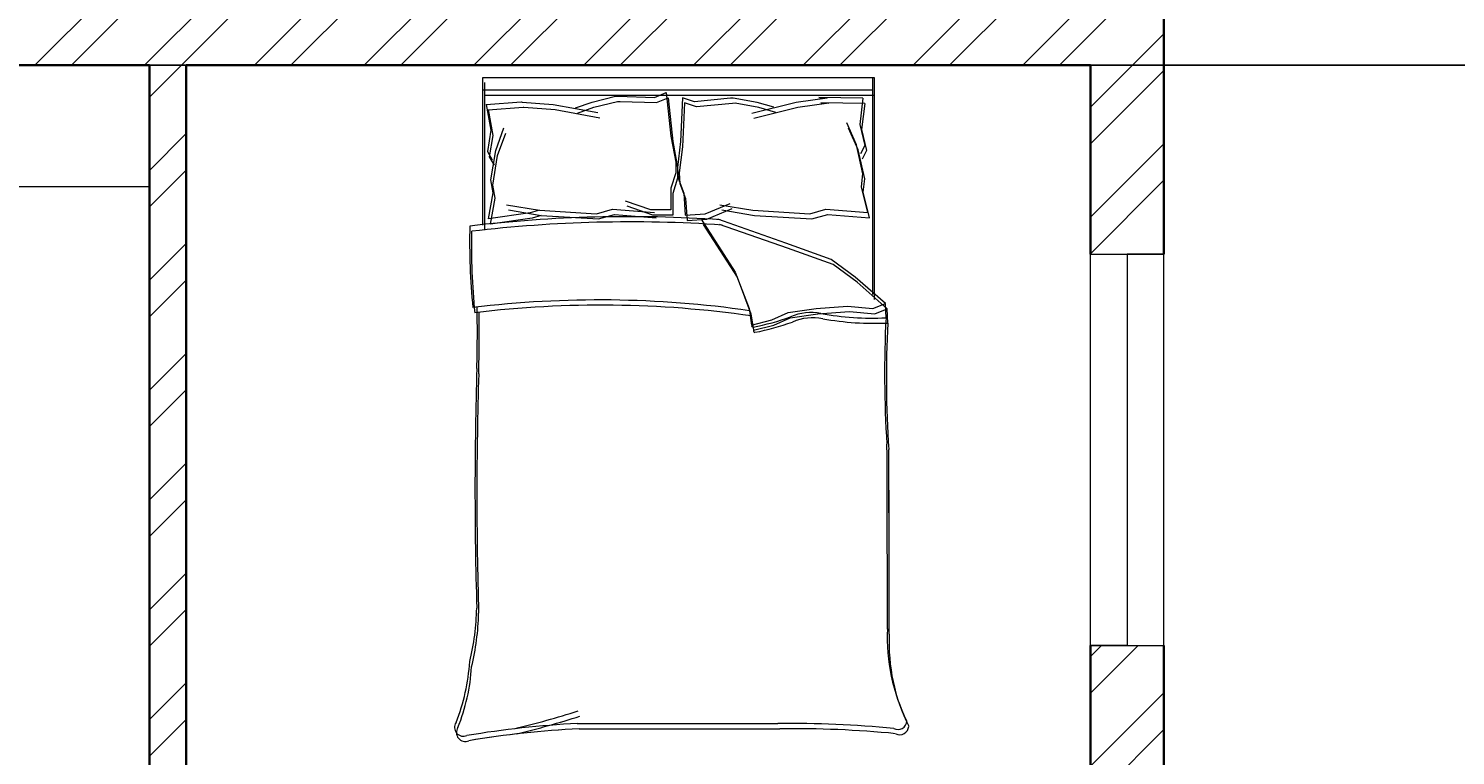
# Model space of a CAD drawing. Units: inches. Extents: x 2552 to 3217, y 1417 to 2737.
# Tile 11 of 25: x 2710 to 2885, y 2302 to 2392. Entities that reach past the tile are written whole.
import ezdxf

# ---------------------------------------------------------------- set-up
doc = ezdxf.new("R2010")
doc.units = ezdxf.units.IN
for name, color, linetype, lineweight in [('A-ANNO-DIMS', 2, 'Continuous', 18), ('A-FLOR-CASE', 9, 'Continuous', 18), ('A-FURN', 8, 'Continuous', 13), ('A-GLAZ', 161, 'Continuous', 18), ('A-WALL', 7, 'Continuous', 35), ('A-WALL-PATT', 217, 'Continuous', 13)]:
    doc.layers.add(name, color=color, linetype=linetype, lineweight=lineweight)
doc.styles.get("Standard").update_dxf_attribs({"font": 'arial.ttf'})
doc.dimstyles.get("Standard").update_dxf_attribs({"dimtxt": 0.18, "dimasz": 0.18, "dimexe": 0.18, "dimexo": 0.0625, "dimgap": 0.09, "dimtad": 0, "dimtih": 1, "dimtoh": 1, "dimdec": 4, "dimzin": 0, "dimdsep": 46, "dimtxsty": 'Standard', "dimcen": 0.09, "dimadec": 0, "dimazin": 0, "dimtfac": 1, "dimtdec": 4, "dimtofl": 0, "dimtmove": 0, "dimatfit": 3, "dimfxl": 1, "dimtolj": 1, "dimtzin": 0, "dimarcsym": 0})

# ---------------------------------------------------------------- blocks, each defined once
blk = doc.blocks.new('BED-DOUBLE')
for p, q in [((3.47, 63.33), (3.47, 81.44)), ((3.47, 81.44), (51.49, 81.44)), ((3.48, 63.33), (3.48, 81.44)), ((3.7, 62.69), (3.7, 80.8)), ((3.7, 62.69), (3.7, 80.8)), ((51.27, 81.44), (51.27, 54.83)), ((51.27, 81.44), (51.27, 54.83)), ((51.49, 81.44), (51.49, 80.8)), ((51.49, 80.8), (51.49, 54.19)), ((51.49, 80.8), (51.49, 54.19)), ((3.47, 79.91), (51.27, 79.91)), ((3.48, 79.91), (51.27, 79.91)), ((3.7, 79.27), (51.49, 79.27)), ((3.7, 79.27), (51.49, 79.27)), ((16.88, 78.42), (19.77, 79.14)), ((16.88, 78.42), (19.77, 79.14)), ((19.77, 79.14), (20.09, 79.14)), ((19.77, 79.14), (20.09, 79.14)), ((20.09, 79.14), (24.54, 78.99)), ((20.09, 79.14), (24.54, 78.99)), ((24.54, 78.99), (25.98, 79.57)), ((24.54, 78.99), (25.98, 79.57)), ((24.77, 78.36), (26.21, 78.93)), ((24.77, 78.36), (26.21, 78.93)), ((25.98, 79.57), (26.56, 74.22)), ((25.98, 79.57), (26.56, 74.22)), ((26.21, 78.93), (26.79, 73.58)), ((26.21, 78.93), (26.79, 73.58)), ((27.98, 78.95), (27.73, 73.58)), ((27.98, 78.95), (27.73, 73.58)), ((29.46, 78.46), (27.98, 78.95)), ((29.46, 78.46), (27.98, 78.95)), ((33.88, 78.89), (29.46, 78.46)), ((33.88, 78.89), (29.46, 78.46)), ((34.2, 78.91), (33.88, 78.89)), ((34.2, 78.91), (33.88, 78.89)), ((37.14, 78.36), (34.2, 78.91)), ((37.14, 78.36), (34.2, 78.91)), ((45.71, 78.9), (41.91, 78.37)), ((45.71, 78.9), (41.91, 78.37)), ((50.11, 78.89), (44.71, 78.98)), ((44.71, 78.98), (45.71, 78.9)), ((50.11, 78.89), (44.71, 78.98)), ((44.71, 78.98), (45.71, 78.9)), ((50.11, 78.89), (49.73, 75.68)), ((50.11, 78.89), (49.73, 75.68)), ((3.89, 78.13), (4.47, 74.95)), ((3.89, 78.13), (4.47, 74.95)), ((3.9, 78.11), (8.18, 78.43)), ((3.9, 78.11), (8.18, 78.43)), ((4.12, 77.49), (4.7, 74.31)), ((4.12, 77.49), (4.7, 74.31)), ((4.13, 77.47), (8.41, 77.8)), ((4.13, 77.47), (8.41, 77.8)), ((8.18, 78.43), (8.28, 78.42)), ((8.18, 78.43), (8.28, 78.42)), ((8.28, 78.42), (12.11, 78.13)), ((8.28, 78.42), (12.11, 78.13)), ((8.41, 77.8), (8.51, 77.78)), ((8.41, 77.8), (8.51, 77.78)), ((8.51, 77.78), (12.34, 77.49)), ((8.51, 77.78), (12.34, 77.49)), ((12.11, 78.13), (17.6, 77.12)), ((12.11, 78.13), (17.6, 77.12)), ((12.34, 77.49), (17.83, 76.48)), ((12.34, 77.49), (17.83, 76.48)), ((14.85, 77.69), (16.88, 78.42)), ((14.85, 77.69), (16.88, 78.42)), ((15.08, 77.05), (17.11, 77.78)), ((15.08, 77.05), (17.11, 77.78)), ((17.11, 77.78), (20, 78.5)), ((17.11, 77.78), (20, 78.5)), ((20, 78.5), (20.32, 78.5)), ((20, 78.5), (20.32, 78.5)), ((20.32, 78.5), (24.77, 78.36)), ((20.32, 78.5), (24.77, 78.36)), ((28.21, 78.31), (27.96, 72.94)), ((28.21, 78.31), (27.96, 72.94)), ((29.68, 77.83), (28.21, 78.31)), ((29.68, 77.83), (28.21, 78.31)), ((34.11, 78.25), (29.68, 77.83)), ((34.11, 78.25), (29.68, 77.83)), ((34.43, 78.27), (34.11, 78.25)), ((34.43, 78.27), (34.11, 78.25)), ((37.36, 77.73), (34.43, 78.27)), ((37.36, 77.73), (34.43, 78.27)), ((41.91, 78.37), (36.49, 77.02)), ((41.91, 78.37), (36.5, 77.02)), ((42.14, 77.73), (36.72, 76.38)), ((42.14, 77.73), (36.72, 76.38)), ((39.2, 77.77), (37.14, 78.36)), ((39.2, 77.77), (37.14, 78.36)), ((39.43, 77.13), (37.36, 77.73)), ((39.43, 77.13), (37.36, 77.73)), ((45.94, 78.26), (42.14, 77.73)), ((45.94, 78.26), (42.14, 77.73)), ((50.34, 78.25), (44.94, 78.34)), ((44.94, 78.34), (45.94, 78.26)), ((50.34, 78.25), (44.94, 78.34)), ((44.94, 78.34), (45.94, 78.26)), ((50.34, 78.25), (49.96, 75.04)), ((50.34, 78.25), (49.96, 75.04)), ((49.31, 73.19), (48.13, 75.86)), ((49.31, 73.19), (48.13, 75.86)), ((49.73, 75.68), (50.33, 73.1)), ((49.73, 75.68), (50.33, 73.1)), ((4.47, 74.95), (4.04, 72.34)), ((4.47, 74.95), (4.04, 72.34)), ((4.7, 74.31), (4.27, 71.7)), ((4.7, 74.31), (4.27, 71.7)), ((5.05, 72.49), (6.06, 75.24)), ((5.05, 72.49), (6.06, 75.24)), ((5.28, 71.85), (6.29, 74.6)), ((5.28, 71.85), (6.29, 74.6)), ((26.56, 74.22), (27.14, 71.04)), ((26.56, 74.22), (27.14, 71.04)), ((26.79, 73.58), (27.37, 70.4)), ((26.79, 73.58), (27.37, 70.4)), ((27.73, 73.58), (27.35, 70.37)), ((27.73, 73.58), (27.35, 70.37)), ((49.54, 72.55), (48.36, 75.23)), ((49.54, 72.55), (48.36, 75.23)), ((49.96, 75.04), (50.56, 72.47)), ((49.96, 75.04), (50.56, 72.47)), ((4.04, 72.34), (4.62, 71.33)), ((4.04, 72.34), (4.62, 71.33)), ((4.47, 68.87), (5.05, 72.49)), ((4.47, 68.87), (5.05, 72.49)), ((4.7, 68.23), (5.28, 71.85)), ((4.7, 68.23), (5.28, 71.85)), ((27.96, 72.94), (27.58, 69.73)), ((27.96, 72.94), (27.58, 69.73)), ((50.11, 69.61), (49.31, 73.19)), ((50.11, 69.61), (49.31, 73.19)), ((50.34, 68.98), (49.54, 72.55)), ((50.34, 68.98), (49.54, 72.55)), ((50.33, 73.1), (49.81, 72.06)), ((50.33, 73.1), (49.81, 72.06)), ((50.56, 72.47), (50.04, 71.42)), ((50.56, 72.47), (50.04, 71.42)), ((4.27, 71.7), (4.85, 70.69)), ((4.27, 71.7), (4.85, 70.69)), ((27.14, 71.04), (27.14, 69.74)), ((27.14, 71.04), (27.14, 69.74)), ((27.35, 70.37), (27.44, 69.07)), ((27.35, 70.37), (27.44, 69.07)), ((27.37, 70.4), (27.37, 69.1)), ((27.37, 70.4), (27.37, 69.1)), ((4.76, 67.28), (4.47, 68.87)), ((4.76, 67.28), (4.47, 68.87)), ((27.14, 69.74), (26.56, 67.86)), ((27.14, 69.74), (26.56, 67.86)), ((27.37, 69.1), (26.79, 67.22)), ((27.37, 69.1), (26.79, 67.22)), ((27.44, 69.07), (28.13, 67.23)), ((27.44, 69.07), (28.13, 67.23)), ((27.58, 69.73), (27.66, 68.43)), ((27.58, 69.73), (27.66, 68.43)), ((27.66, 68.43), (28.36, 66.59)), ((27.66, 68.43), (28.36, 66.59)), ((49.92, 68.01), (50.11, 69.61)), ((49.92, 68.01), (50.11, 69.61)), ((50.15, 67.37), (50.34, 68.98)), ((50.15, 67.37), (50.34, 68.98)), ((4.18, 64.1), (4.76, 67.28)), ((4.18, 64.1), (4.76, 67.28)), ((4.41, 63.46), (4.99, 66.64)), ((4.41, 63.46), (4.99, 66.64)), ((4.99, 66.64), (4.7, 68.23)), ((4.99, 66.64), (4.7, 68.23)), ((26.56, 67.86), (26.56, 65.18)), ((26.56, 67.86), (26.56, 65.18)), ((26.79, 67.22), (26.79, 64.54)), ((26.79, 67.22), (26.79, 64.54)), ((28.13, 67.23), (28.3, 64.55)), ((28.13, 67.23), (28.3, 64.55)), ((28.36, 66.59), (28.53, 63.91)), ((28.36, 66.59), (28.53, 63.91)), ((50.7, 64.87), (49.92, 68.01)), ((50.7, 64.87), (49.92, 68.01)), ((50.93, 64.23), (50.15, 67.37)), ((50.93, 64.23), (50.15, 67.37)), ((9.28, 64.83), (4.18, 64.1)), ((9.28, 64.83), (4.18, 64.1)), ((6.38, 65.81), (10.41, 65.15)), ((6.38, 65.81), (10.41, 65.15)), ((6.61, 65.18), (10.64, 64.51)), ((6.61, 65.18), (10.64, 64.51)), ((10.41, 65.15), (9.28, 64.83)), ((10.41, 65.15), (9.28, 64.83)), ((10.41, 65.15), (17.42, 64.72)), ((10.41, 65.15), (17.42, 64.72)), ((17.42, 64.72), (19.38, 65.27)), ((17.42, 64.72), (19.38, 65.27)), ((19.38, 65.27), (24.52, 64.87)), ((19.38, 65.27), (24.52, 64.87)), ((24.1, 65.18), (20.96, 66.27)), ((24.1, 65.18), (20.96, 66.27)), ((24.33, 64.54), (21.19, 65.63)), ((24.33, 64.54), (21.19, 65.63)), ((26.56, 65.18), (24.1, 65.18)), ((26.56, 65.18), (24.1, 65.18)), ((30.75, 64.7), (33.82, 65.99)), ((30.75, 64.7), (33.82, 65.99)), ((30.98, 64.06), (34.05, 65.35)), ((30.98, 64.06), (34.05, 65.35)), ((32.56, 65.81), (36.6, 65.15)), ((32.56, 65.81), (36.6, 65.15)), ((32.79, 65.18), (36.82, 64.51)), ((32.79, 65.18), (36.82, 64.51)), ((36.6, 65.15), (43.61, 64.72)), ((36.6, 65.15), (43.61, 64.72)), ((43.61, 64.72), (45.57, 65.27)), ((43.61, 64.72), (45.57, 65.27)), ((45.57, 65.27), (50.7, 64.87)), ((45.57, 65.27), (50.7, 64.87)), ((9.51, 64.19), (4.41, 63.46)), ((9.51, 64.19), (4.41, 63.46)), ((10.64, 64.51), (9.51, 64.19)), ((10.64, 64.51), (9.51, 64.19)), ((10.64, 64.51), (17.65, 64.08)), ((10.64, 64.51), (17.65, 64.08)), ((17.65, 64.08), (19.61, 64.63)), ((17.65, 64.08), (19.61, 64.63)), ((19.61, 64.63), (24.74, 64.23)), ((19.61, 64.63), (24.74, 64.23)), ((26.79, 64.54), (24.33, 64.54)), ((26.79, 64.54), (24.33, 64.54)), ((28.3, 64.55), (30.75, 64.7)), ((28.3, 64.55), (30.75, 64.7)), ((28.53, 63.91), (30.98, 64.06)), ((28.53, 63.91), (30.98, 64.06)), ((30.26, 64.06), (34.45, 57.57)), ((30.26, 64.06), (34.45, 57.57)), ((30.49, 63.42), (34.68, 56.93)), ((30.49, 63.42), (34.68, 56.93)), ((40.64, 61.13), (32.31, 64.06)), ((40.64, 61.13), (32.31, 64.06)), ((40.87, 60.49), (32.53, 63.42)), ((40.87, 60.49), (32.53, 63.42)), ((36.82, 64.51), (43.83, 64.08)), ((36.82, 64.51), (43.83, 64.08)), ((43.83, 64.08), (45.79, 64.63)), ((43.83, 64.08), (45.79, 64.63)), ((45.79, 64.63), (50.93, 64.23)), ((45.79, 64.63), (50.93, 64.23)), ((46.22, 59.11), (40.64, 61.13)), ((46.22, 59.11), (40.64, 61.13)), ((46.45, 58.48), (40.87, 60.49)), ((46.45, 58.48), (40.87, 60.49)), ((49.16, 56.95), (46.22, 59.11)), ((49.16, 56.95), (46.22, 59.11)), ((49.39, 56.31), (46.45, 58.48)), ((49.39, 56.31), (46.45, 58.48)), ((34.45, 57.57), (36.15, 53.08)), ((34.45, 57.57), (36.15, 53.08)), ((34.68, 56.93), (36.38, 52.44)), ((34.68, 56.93), (36.38, 52.44)), ((52.87, 53.7), (49.16, 56.95)), ((52.87, 53.7), (49.16, 56.95)), ((53.1, 53.06), (49.39, 56.31)), ((53.1, 53.06), (49.39, 56.31)), ((36.15, 53.08), (36.46, 51.07)), ((36.15, 53.08), (36.46, 51.07)), ((38.94, 51.69), (40.95, 52.61)), ((38.94, 51.69), (40.95, 52.61)), ((40.95, 52.61), (44.36, 53.08)), ((40.95, 52.61), (44.36, 53.08)), ((44.36, 53.08), (48.23, 53.39)), ((44.36, 53.08), (48.23, 53.39)), ((44.59, 52.44), (48.46, 52.75)), ((44.59, 52.44), (48.46, 52.75)), ((48.23, 53.39), (51.33, 53.08)), ((48.23, 53.39), (51.33, 53.08)), ((48.46, 52.75), (51.56, 52.44)), ((48.46, 52.75), (51.56, 52.44)), ((51.33, 53.08), (52.87, 53.7)), ((51.33, 53.08), (52.87, 53.7)), ((51.56, 52.44), (53.1, 53.06)), ((51.56, 52.44), (53.1, 53.06)), ((52.95, 51.95), (52.87, 53.7, 3.87)), ((52.95, 51.95), (52.87, 53.7, 3.87)), ((53.18, 51.31), (53.1, 53.06, 3.87)), ((53.18, 51.31), (53.1, 53.06, 3.87)), ((36.38, 52.44), (36.69, 50.43)), ((36.38, 52.44), (36.69, 50.43)), ((36.46, 51.07), (38.94, 51.69)), ((36.46, 51.07), (38.94, 51.69)), ((36.69, 50.43), (39.17, 51.05)), ((36.69, 50.43), (39.17, 51.05)), ((39.17, 51.05), (41.18, 51.97)), ((39.17, 51.05), (41.18, 51.97)), ((41.18, 51.97), (44.59, 52.44)), ((41.18, 51.97), (44.59, 52.44)), ((15.06, 2.2), (39.68, 2.2)), ((15.06, 2.2), (39.68, 2.2)), ((15.29, 1.56), (39.91, 1.56)), ((15.29, 1.56), (39.91, 1.56))]:
    blk.add_line(p, q)
for centre, radius, start, end in [((85.16, 61.35), 83.31, 178.7218, 185.604), ((85.16, 61.35), 83.31, 178.7218, 185.604), ((21.36, -100.61), 164.97, 86.0865, 96.7821), ((21.36, -100.61), 164.97, 86.0865, 96.7821), ((21.59, -101.25), 164.97, 86.0865, 96.7821), ((21.59, -101.25), 164.97, 86.0865, 96.7821), ((85.39, 60.71), 83.31, 178.7218, 185.604), ((85.39, 60.71), 83.31, 178.7218, 185.604), ((17.76, -74.87), 129.02, 81.7845, 96.9006), ((17.76, -74.87), 129.02, 81.7845, 96.9006), ((17.98, -75.51), 129.02, 81.7845, 96.9006), ((17.98, -75.51), 129.02, 81.7845, 96.9006), ((-167.31, 50.27), 170.11, 358.4762, 1.0082), ((-167.31, 50.27), 170.11, 358.4762, 1.0082), ((-167.08, 49.63), 170.11, 358.4762, 1.0082), ((-167.08, 49.63), 170.11, 358.4762, 1.0082), ((43.74, 46.38), 6.22, 78.6608, 113.7384), ((43.74, 46.38), 6.22, 78.6608, 113.7384), ((36.64, 51), 0.185, 160.2464, 271.1377), ((36.64, 51), 0.185, 160.2464, 271.1377), ((31.15, 79.96), 29.65, 280.6617, 289.8806), ((31.15, 79.96), 29.65, 280.6617, 289.8806), ((31.38, 79.32), 29.65, 280.6617, 289.8806), ((31.38, 79.32), 29.65, 280.6617, 289.8806), ((43.97, 45.74), 6.22, 78.6608, 113.7384), ((43.97, 45.74), 6.22, 78.6608, 113.7384), ((51.33, 88.1), 36.18, 259.8763, 272.5657), ((51.33, 88.1), 36.18, 259.8763, 272.5657), ((51.56, 87.46), 36.18, 259.8763, 272.5657), ((51.56, 87.46), 36.18, 259.8763, 272.5657), ((182.27, 45.13), 129.5, 176.9791, 183.8365), ((182.27, 45.13), 129.5, 176.9791, 183.8365), ((182.49, 44.49), 129.5, 176.9791, 183.8365), ((182.49, 44.49), 129.5, 176.9791, 183.8365), ((36.86, 50.36), 0.185, 160.2464, 271.1377), ((36.86, 50.36), 0.185, 160.2464, 271.1377), ((484.82, 30.83), 482.31, 178.2277, 181.7185), ((484.82, 30.83), 482.31, 178.2277, 181.7185), ((485.05, 30.19), 482.31, 178.2277, 181.7185), ((485.05, 30.19), 482.31, 178.2277, 181.7185), ((-4508.74, 13.62), 4561.86, 0.00217, 0.28689), ((-4508.74, 13.62), 4561.86, 0.00217, 0.28689), ((-4508.51, 12.98), 4561.86, 0.00217, 0.28689), ((-4508.52, 12.98), 4561.86, 0.00217, 0.28689), ((-26.9, 16.93), 29.63, 346.0648, 358.9113), ((-26.9, 16.93), 29.63, 346.0648, 358.9113), ((-26.67, 16.29), 29.63, 346.0648, 358.9113), ((-26.67, 16.29), 29.63, 346.0648, 358.9113), ((76.16, 12.78), 23.07, 177.4714, 206.4681), ((76.16, 12.78), 23.07, 177.4714, 206.4681), ((76.39, 12.14), 23.07, 177.4714, 206.4681), ((76.39, 12.14), 23.07, 177.4714, 206.4681), ((-21.66, 11.17), 23.56, 337.9751, 356.652), ((-21.66, 11.17), 23.56, 337.9751, 356.652), ((-21.43, 10.53), 23.56, 337.9751, 356.652), ((-21.43, 10.53), 23.56, 337.9751, 356.652), ((-17.22, 105.16), 106.46, 283.3832, 287.7053), ((-17.22, 105.16), 106.46, 283.3832, 287.7053), ((1.09, 1.73), 1.09, 146.1736, 293.4781), ((1.09, 1.73), 1.09, 146.1736, 293.4781), ((21.43, -119.39), 121.76, 92.9958, 99.4091), ((21.43, -119.39), 121.76, 92.9958, 99.4091), ((-16.99, 104.52), 106.46, 283.3832, 287.7053), ((-16.99, 104.52), 106.46, 283.3832, 287.7053), ((41.15, -130.83), 133.04, 84.4998, 90.6351), ((41.15, -130.83), 133.04, 84.4998, 90.6351), ((54.41, 2.57), 1.1, 242.6588, 356.02), ((54.41, 2.57), 1.1, 242.6588, 356.02), ((54.64, 1.93), 1.1, 242.6588, 356.02), ((54.64, 1.93), 1.1, 242.6588, 356.02), ((1.32, 1.09), 1.09, 146.1736, 293.4781), ((1.32, 1.09), 1.09, 146.1736, 293.4781), ((21.66, -120.03), 121.76, 92.9958, 99.4091), ((21.65, -120.03), 121.76, 92.9958, 99.4091), ((41.38, -131.47), 133.04, 84.4998, 90.6351), ((41.38, -131.47), 133.04, 84.4998, 90.6351)]:
    blk.add_arc(centre, radius, start, end)
blk = doc.blocks.new('WIN-48')
for p, q in [((4.5, 48), (0, 48)), ((0, 48), (9, 48)), ((0, 48), (0, 0)), ((4.5, 0), (4.5, 48)), ((9, 48), (9, 0)), ((0, 0), (9, 0)), ((9, 0), (4.5, 0))]:
    blk.add_line(p, q)
blk = doc.blocks.new('*D64')
at = {"layer": 'A-ANNO-DIMS', "color": 0, "lineweight": -2, "transparency": 16777216}
for p, q in [((2646.35, 1551.58), (2646.35, 2709.49)), ((2646.53, 2709.31), (2802.77, 2709.31)), ((2959.93, 2709.31), (2803.69, 2709.31)), ((2960.11, 1551.58), (2960.11, 2709.49))]:
    blk.add_line(p, q, dxfattribs=at)
at = {"layer": 'A-ANNO-DIMS', "color": 0, "transparency": 16777216}
for points in [[(2646.53, 2709.34), (2646.53, 2709.28), (2646.35, 2709.31)], [(2959.93, 2709.34), (2959.93, 2709.28), (2960.11, 2709.31)]]:
    blk.add_solid(points, dxfattribs=at)
at = {"layer": 'Defpoints', "color": 0, "transparency": 16777216}
for p in [(2960.11, 2709.31), (2646.35, 1551.51), (2960.11, 1551.51)]:
    blk.add_point(p, dxfattribs=at)
at = {"layer": 'A-ANNO-DIMS', "color": 0, "transparency": 16777216, "insert": (2803.23, 2709.31), "char_height": 0.18, "attachment_point": 5}
blk.add_mtext('\\A1;313.76', dxfattribs=at)
blk = doc.blocks.new('*D69')
at = {"layer": 'A-ANNO-DIMS', "color": 0, "lineweight": -2, "transparency": 16777216}
for p, q in [((2908.79, 2403.41), (2577.37, 2403.41)), ((2577.55, 2403.23), (2577.55, 2395.39)), ((2577.55, 2387.19), (2577.55, 2395.03)), ((2917.79, 2387.01), (2577.37, 2387.01))]:
    blk.add_line(p, q, dxfattribs=at)
at = {"layer": 'A-ANNO-DIMS', "color": 0, "transparency": 16777216}
for points in [[(2577.52, 2403.23), (2577.58, 2403.23), (2577.55, 2403.41)], [(2577.52, 2387.19), (2577.58, 2387.19), (2577.55, 2387.01)]]:
    blk.add_solid(points, dxfattribs=at)
at = {"layer": 'Defpoints', "color": 0, "transparency": 16777216}
for p in [(2577.55, 2403.41), (2908.85, 2403.41), (2917.85, 2387.01)]:
    blk.add_point(p, dxfattribs=at)
at = {"layer": 'A-ANNO-DIMS', "color": 0, "transparency": 16777216, "insert": (2577.55, 2395.21), "char_height": 0.18, "attachment_point": 5}
blk.add_mtext('\\A1;16.4', dxfattribs=at)

msp = doc.modelspace()

# ---------------------------------------------------------------- hatches: boundary and pattern name
at = {"layer": 'A-WALL-PATT'}
h = msp.add_hatch(dxfattribs=at)
h.set_pattern_fill('ANSI32', color=256)
h.paths.add_polyline_path([(2756.676, 2649.5125), (2637.3535, 2649.5125), (2637.3535, 2617.9626), (2641.8535, 2617.9626), (2646.3535, 2617.9626), (2646.3535, 2640.5125), (2724.3535, 2640.5125), (2724.3535, 2520.5125), (2720.299, 2520.5125), (2720.299, 2516.0125), (2733.4075, 2516.0125), (2733.4075, 2518.2213), (2733.4075, 2520.5125), (2728.8535, 2520.5125), (2728.8535, 2640.5125), (2756.676, 2640.5125)])
h.paths.add_polyline_path([(2848.8535, 2649.5125), (2804.676, 2649.5125), (2804.676, 2640.5125), (2839.8535, 2640.5125), (2839.8535, 2598.3517), (2848.8535, 2598.3517)])
h.paths.add_polyline_path([(2646.3535, 2516.0125), (2697.9593, 2516.0125), (2697.9593, 2518.2625), (2697.9593, 2520.5125), (2646.3535, 2520.5125), (2646.3535, 2581.9626), (2637.3535, 2581.9626), (2637.3535, 2364.3298), (2646.3535, 2364.3298), (2646.3535, 2387.0125), (2724.3535, 2387.0125), (2724.3535, 2267.0125), (2721.0443, 2267.0125), (2721.0443, 2262.5125), (2733.7854, 2262.5125), (2733.7854, 2264.7625), (2733.7854, 2267.0125), (2728.8535, 2267.0125), (2728.8535, 2387.0125), (2839.8535, 2387.0125), (2839.8535, 2363.8387), (2848.8535, 2363.8387), (2848.8535, 2403.7415), (2844.3535, 2403.7415), (2839.8535, 2403.7415), (2839.8535, 2396.0125), (2646.3535, 2396.0125)])
h.paths.add_polyline_path([(2848.8535, 2550.3517), (2844.3535, 2550.3517), (2839.8535, 2550.3517), (2839.8535, 2520.5125), (2801.9195, 2520.5125), (2801.9195, 2518.2625), (2801.9195, 2516.0125), (2839.8535, 2516.0125), (2839.8535, 2507.5813), (2848.8535, 2507.5813)], flags=17)
h.paths.add_polyline_path([(2848.8535, 2483.5813), (2844.3535, 2483.5813), (2839.8535, 2483.5813), (2839.8535, 2468.0125), (2773.8535, 2468.0125), (2773.8535, 2516.0125), (2778.1336, 2516.0125), (2778.1336, 2520.5125), (2766.696, 2520.5125), (2766.696, 2518.2625), (2766.696, 2516.0125), (2769.3535, 2516.0125), (2769.3535, 2463.5125), (2839.8535, 2463.5125), (2839.8535, 2431.0782), (2848.8535, 2431.0782)], flags=17)
h.paths.add_polyline_path([(2917.8535, 2569.2764), (2913.3535, 2569.2764), (2908.8535, 2569.2764), (2908.8535, 2433.001), (2917.8535, 2433.001), (2917.8535, 2516.0125), (2967.486, 2516.0125), (2967.486, 2520.5125), (2917.8535, 2520.5125)])
h.paths.add_polyline_path([(3000.3535, 2640.5125), (2995.8535, 2640.5125), (2995.8535, 2520.5125), (2990.688, 2520.5125), (2990.688, 2516.0125), (3004.0844, 2516.0125), (3004.0844, 2518.2625), (3004.0844, 2520.5125), (3000.3535, 2520.5125)])
h.paths.add_polyline_path([(3120.3535, 2561.3689), (3115.8535, 2561.3689), (3111.3535, 2561.3689), (3111.3535, 2520.5125), (3070.9814, 2520.5125), (3070.9814, 2518.2625), (3070.9814, 2516.0125), (3111.3535, 2516.0125), (3111.3535, 2505.1841), (3120.3535, 2505.1841)])
h.paths.add_polyline_path([(3120.3535, 2481.1841), (3115.8535, 2481.1841), (3111.3535, 2481.1841), (3111.3535, 2468.0125), (3045.3535, 2468.0125), (3045.3535, 2516.0125), (3048.9787, 2516.0125), (3048.9787, 2520.5125), (3036.3395, 2520.5125), (3036.3395, 2516.0125), (3040.8535, 2516.0125), (3040.8535, 2463.5125), (3111.3535, 2463.5125), (3111.3535, 2396.0125), (2917.8535, 2396.0125), (2917.8535, 2403.4124), (2913.3535, 2403.4124), (2908.8535, 2403.4124), (2908.8535, 2182.5756), (2917.8535, 2182.5756), (2917.8535, 2262.5125), (2968.001, 2262.5125), (2968.001, 2264.7625), (2968.001, 2267.0125), (2917.8535, 2267.0125), (2917.8535, 2387.0125), (3111.3535, 2387.0125), (3111.3535, 2352.2435), (3120.3535, 2352.2435)])
h.paths.add_polyline_path([(3120.3535, 2304.2435), (3115.8535, 2304.2435), (3111.3535, 2304.2435), (3111.3535, 2267.0125), (3073.8616, 2267.0125), (3073.8616, 2264.7625), (3073.8616, 2262.5125), (3111.3535, 2262.5125), (3111.3535, 2252.376), (3120.3535, 2252.376)], flags=17)
h.paths.add_polyline_path([(3120.3535, 2228.376), (3115.8535, 2228.376), (3111.3535, 2228.376), (3111.3535, 2214.5125), (3045.3535, 2214.5125), (3045.3535, 2262.5125), (3049.3096, 2262.5125), (3049.3096, 2267.0125), (3035.0125, 2267.0125), (3035.0125, 2262.5125), (3040.8535, 2262.5125), (3040.8535, 2210.0125), (3111.3535, 2210.0125), (3111.3535, 2142.5125), (2917.8535, 2142.5125), (2917.8535, 2150.2408), (2913.3535, 2150.2408), (2908.8535, 2150.2408), (2908.8535, 1924.9905), (2917.8535, 1924.9905), (2917.8535, 2009.0125), (2971.959, 2009.0125), (2971.959, 2011.2625), (2971.959, 2013.5125), (2917.8535, 2013.5125), (2917.8535, 2133.5125), (2995.8535, 2133.5125), (2995.8535, 2013.5125), (2992.1797, 2013.5125), (2992.1797, 2009.0125), (3004.3344, 2009.0125), (3004.3344, 2011.2625), (3004.3344, 2013.5125), (3000.3535, 2013.5125), (3000.3535, 2133.5125), (3111.3535, 2133.5125), (3111.3535, 2115.0291), (3120.3535, 2115.0291)])
h.paths.add_polyline_path([(3000.3535, 2387.0125), (2995.8535, 2387.0125), (2995.8535, 2267.0125), (2991.3326, 2267.0125), (2991.3326, 2262.5125), (3004.1044, 2262.5125), (3004.1044, 2264.7625), (3004.1044, 2267.0125), (3000.3535, 2267.0125)], flags=17)
h.paths.add_polyline_path([(3120.3535, 1973.2388), (3115.8535, 1973.2388), (3111.3535, 1973.2388), (3111.3535, 1961.0125), (3045.3535, 1961.0125), (3045.3535, 2009.0125), (3048.9101, 2009.0125), (3048.9101, 2013.5125), (3037.105, 2013.5125), (3037.105, 2011.2625), (3037.105, 2009.0125), (3040.8535, 2009.0125), (3040.8535, 1956.5125), (3111.3535, 1956.5125), (3111.3535, 1889.0125), (2917.8535, 1889.0125), (2917.8535, 1895.7215), (2913.3535, 1895.7215), (2908.8535, 1895.7215), (2908.8535, 1844.2217), (2917.8535, 1844.2217), (2917.8535, 1880.0125), (3111.3535, 1880.0125), (3111.3535, 1846.9541), (3120.3535, 1846.9541)])
h.paths.add_polyline_path([(3120.3535, 2067.0291), (3111.3535, 2067.0291), (3111.3535, 2013.5125), (3071.3001, 2013.5125), (3071.3001, 2009.0125), (3111.3535, 2009.0125), (3111.3535, 1997.2388), (3120.3535, 1997.2388)], flags=0)
h.paths.add_polyline_path([(3120.3535, 1798.9541), (3115.8535, 1798.9541), (3111.3535, 1798.9541), (3111.3535, 1760.0125), (3071.2497, 1760.0125), (3071.2497, 1757.7625), (3071.2497, 1755.5125), (3111.3535, 1755.5125), (3111.3535, 1746.162), (3120.3535, 1746.2478)])
h.paths.add_polyline_path([(3120.3535, 1722.2049), (3111.3535, 1722.2049), (3111.3535, 1707.5125), (3045.3535, 1707.5125), (3045.3535, 1755.5125), (3048.6624, 1755.5125), (3048.6624, 1760.0125), (3035.3703, 1760.0125), (3035.3703, 1755.5125), (3040.8535, 1755.5125), (3040.8535, 1703.0125), (3111.3535, 1703.0125), (3111.3535, 1635.5125), (2917.8535, 1635.5125), (2917.8535, 1643.1366), (2913.3535, 1643.1366), (2908.8535, 1643.1366), (2908.8535, 1626.5125), (3120.3535, 1626.5125)])
h.paths.add_polyline_path([(2917.8535, 1755.5125), (2973.2287, 1755.5125), (2973.2287, 1757.7625), (2973.2287, 1760.0125), (2917.8535, 1760.0125), (2917.8535, 1808.2217), (2913.3535, 1808.2217), (2908.8535, 1808.2217), (2908.8535, 1676.1665), (2917.8535, 1676.1665)])
h.paths.add_polyline_path([(3000.3535, 1880.0125), (2995.8535, 1880.0125), (2995.8535, 1760.0125), (2992.9329, 1760.0125), (2992.9329, 1755.5125), (3003.8766, 1755.5125), (3003.8766, 1757.7625), (3003.8766, 1760.0125), (3000.3535, 1760.0125)])
h.paths.add_polyline_path([(2848.8535, 1896.6971), (2844.3535, 1896.6971), (2839.8535, 1896.6971), (2839.8535, 1889.0125), (2646.3535, 1889.0125), (2646.3535, 2009.0125), (2700.5253, 2009.0125), (2700.5253, 2011.2625), (2700.5253, 2013.5125), (2646.3535, 2013.5125), (2646.3535, 2053.1812), (2641.8535, 2053.1812), (2637.3535, 2053.1812), (2637.3535, 1836.254), (2646.3535, 1836.254), (2646.3535, 1880.0125), (2724.3535, 1880.0125), (2724.3535, 1760.0125), (2721.2473, 1760.0125), (2721.2473, 1755.5125), (2731.9187, 1755.5125), (2731.9187, 1757.7625), (2731.9187, 1760.0125), (2728.8535, 1760.0125), (2728.8535, 1880.0125), (2839.8535, 1880.0125), (2839.8535, 1840.3813), (2848.8535, 1840.3813)])
h.paths.add_polyline_path([(2848.8535, 1792.3813), (2844.3535, 1792.3813), (2839.8535, 1792.3813), (2839.8535, 1760.0125), (2797.8845, 1760.0125), (2797.8845, 1755.5125), (2839.8535, 1755.5125), (2839.8535, 1743.3688), (2844.3535, 1743.3688), (2848.8535, 1743.3688)], flags=0)
h.paths.add_polyline_path([(2848.8535, 1719.3688), (2844.3535, 1719.3688), (2839.8535, 1719.3688), (2839.8535, 1707.5125), (2773.8535, 1707.5125), (2773.8535, 1755.5125), (2777.716, 1755.5125), (2777.716, 1760.0125), (2760.9247, 1760.0125), (2760.9247, 1757.9721), (2760.9247, 1755.5125), (2769.3535, 1755.5125), (2769.3535, 1703.0125), (2839.8535, 1703.0125), (2839.8535, 1673.0277), (2848.8535, 1672.9407)], flags=0)
h.paths.add_polyline_path([(2646.3535, 1755.5125), (2702.9171, 1755.5125), (2702.9171, 1757.7625), (2702.9171, 1760.0125), (2646.3535, 1760.0125), (2646.3535, 1800.254), (2641.8535, 1800.254), (2637.3535, 1800.254), (2637.3535, 1626.5125), (2848.8535, 1626.5125), (2848.8535, 1643.1187), (2844.3535, 1643.1187), (2839.8535, 1643.1187), (2839.8535, 1635.5125), (2646.3535, 1635.5125)])
h.paths.add_polyline_path([(2848.8535, 2148.8427), (2844.3535, 2148.8427), (2839.8535, 2148.8427), (2839.8535, 2142.5125), (2646.3535, 2142.5125), (2646.3535, 2262.5125), (2701.3562, 2262.5125), (2701.3562, 2264.7625), (2701.3562, 2267.0125), (2646.3535, 2267.0125), (2646.3535, 2328.3298), (2637.3535, 2328.3298), (2637.3535, 2089.1812), (2646.3535, 2089.1812), (2646.3535, 2133.5125), (2839.8535, 2133.5125), (2839.8535, 2097.5966), (2848.8535, 2097.5966)])
h.paths.add_polyline_path([(2728.8535, 2133.5125), (2724.3535, 2133.5125), (2724.3535, 2013.5125), (2719.6039, 2013.5125), (2719.6039, 2009.0125), (2732.5784, 2009.0125), (2732.5784, 2011.2625), (2732.5784, 2013.5125), (2728.8535, 2013.5125)])
h.paths.add_polyline_path([(2848.8535, 1970.0557), (2844.3535, 1970.0557), (2839.8535, 1970.0557), (2839.8535, 1961.0125), (2773.8535, 1961.0125), (2773.8535, 2009.0125), (2777.3388, 2009.0125), (2777.3388, 2013.5125), (2764.7681, 2013.5125), (2764.7681, 2009.0125), (2769.3535, 2009.0125), (2769.3535, 1956.5125), (2839.8535, 1956.5125), (2839.8535, 1924.7199), (2848.8535, 1924.7199)], flags=17)
h.paths.add_polyline_path([(2848.8535, 2049.5966), (2844.3535, 2049.5966), (2839.8535, 2049.5966), (2839.8535, 2013.5125), (2798.198, 2013.5125), (2798.198, 2011.2625), (2798.198, 2009.0125), (2839.8535, 2009.0125), (2839.8535, 1994.0557), (2848.8535, 1994.0557)], flags=17)
h.paths.add_polyline_path([(2848.8535, 2315.8387), (2839.8535, 2315.8387), (2839.8535, 2267.0125), (2799.3375, 2267.0125), (2799.3375, 2264.7625), (2799.3375, 2262.5125), (2839.8535, 2262.5125), (2839.8535, 2253.2843), (2848.8535, 2253.2843)], flags=17)
h.paths.add_polyline_path([(2848.8535, 2229.2843), (2839.8535, 2229.2843), (2839.8535, 2177.6936), (2848.8535, 2177.6936)], flags=17)
h.paths.add_polyline_path([(2839.8535, 2214.5125), (2773.8535, 2214.5125), (2773.8535, 2262.5125), (2777.6984, 2262.5125), (2777.6984, 2267.0125), (2763.8226, 2267.0125), (2763.8226, 2262.5125), (2769.3535, 2262.5125), (2769.3535, 2210.0125), (2839.8535, 2210.0125)], flags=17)
h.paths.add_polyline_path([(3050.32, 2520.2817), (3088.9114, 2520.2817), (3088.9114, 2538.939), (3050.32, 2538.939)], flags=9)

# ---------------------------------------------------------------- linework, layer by layer
at = {"layer": 'A-FLOR-CASE'}
for p in [(2662.3425, 2372.1585), (2724.3535, 2372.1585)]:
    msp.add_line(p, (2724.3535, 2372.1585), dxfattribs=at)
at = {"layer": 'A-WALL'}
for p, q in [((2848.8535, 2403.7415), (2848.8535, 2363.8387)), ((2646.3535, 2387.0125), (2724.3535, 2387.0125)), ((2724.3535, 2387.0125), (2724.3535, 2267.0125)), ((2728.8535, 2387.0125), (2728.8535, 2267.0125)), ((2728.8535, 2387.0125), (2839.8535, 2387.0125)), ((2839.8535, 2387.0125), (2839.8535, 2363.8387)), ((2839.8535, 2315.8387), (2839.8535, 2267.0125)), ((2848.8535, 2315.8387), (2848.8535, 2253.2843))]:
    msp.add_line(p, q, dxfattribs=at)

# ---------------------------------------------------------------- block references
at = {"layer": 'A-FURN'}
msp.add_blockref('BED-DOUBLE', (2761.804, 2304.0828), dxfattribs=at)
at = {"layer": 'A-GLAZ', "extrusion": (0, 0, -1), "zscale": -1, "rotation": 180}
msp.add_blockref('WIN-48', (-2839.854, 2363.8383), dxfattribs=at)

# ---------------------------------------------------------------- dimensions: what is measured, and where the dimension line sits
at = {"layer": 'A-ANNO-DIMS'}
dim = msp.add_linear_dim(base=(2960.1089, 2709.3125), p1=(2646.3535, 1551.5125), p2=(2960.1089, 1551.5125), dimstyle='Standard', override={"dimdec": 2, "dimlfac": 1, "dimrnd": 0, "dimzin": 0, "dimdsep": 46, "dimlunit": 2}, dxfattribs=at)
dim.commit()
dim.dimension.update_dxf_attribs({"geometry": '*D64', "text_midpoint": (2803.2312, 2709.3125)})
dim = msp.add_linear_dim(base=(2577.5535, 2403.4124), p1=(2917.8535, 2387.0125), p2=(2908.8535, 2403.4124), angle=90, dimstyle='Standard', override={"dimdec": 1, "dimlfac": 1, "dimrnd": 0, "dimzin": 0, "dimdsep": 46, "dimlunit": 2}, dxfattribs=at)
dim.commit()
dim.dimension.update_dxf_attribs({"geometry": '*D69', "text_midpoint": (2577.5535, 2395.2125)})

doc.saveas('drawing.dxf')
